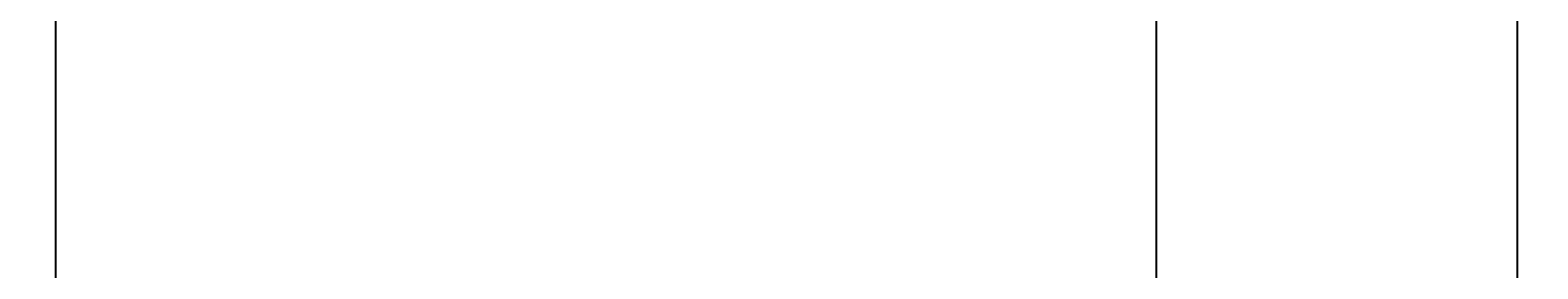
# Model space of a CAD drawing. Units: inches. Extents: x 35362 to 73946, y 43607 to 67532.
# Tile 77 of 134: x 50119 to 51337, y 46919 to 47112. Entities that reach past the tile are written whole.
import ezdxf

# ---------------------------------------------------------------- set-up
doc = ezdxf.new("R2010")
doc.units = ezdxf.units.IN
doc.header["$MEASUREMENT"] = 0
doc.layers.add('A-ANNO-DIMS', color=2, linetype='Continuous', lineweight=18)
doc.styles.get("Standard").update_dxf_attribs({"font": 'arial.ttf'})
doc.dimstyles.get("Standard").update_dxf_attribs({"dimtxt": 0.18, "dimasz": 0.18, "dimexe": 0.18, "dimexo": 0.0625, "dimgap": 0.09, "dimtad": 0, "dimtih": 1, "dimtoh": 1, "dimdec": 4, "dimzin": 0, "dimdsep": 46, "dimtxsty": 'Standard', "dimcen": 0.09, "dimadec": 0, "dimazin": 0, "dimtfac": 1, "dimtdec": 4, "dimtofl": 0, "dimtmove": 0, "dimatfit": 3, "dimfxl": 1, "dimtolj": 1, "dimtzin": 0, "dimarcsym": 0})

# ---------------------------------------------------------------- blocks, each defined once
blk = doc.blocks.new('*D11')
at = {"layer": 'A-ANNO-DIMS', "color": 0, "lineweight": -2, "transparency": 16777216}
for p, q in [((47978.7, 56028.8), (47978.7, 43606.7)), ((53109.8, 56028.8), (53109.8, 43606.7)), ((47978.8, 43606.9), (50543.9, 43606.9)), ((53109.6, 43606.9), (50544.6, 43606.9))]:
    blk.add_line(p, q, dxfattribs=at)
at = {"layer": 'A-ANNO-DIMS', "color": 0, "transparency": 16777216}
for points in [[(47978.8, 43606.9), (47978.8, 43606.8), (47978.7, 43606.9)], [(53109.6, 43606.9), (53109.6, 43606.8), (53109.8, 43606.9)]]:
    blk.add_solid(points, dxfattribs=at)
at = {"layer": 'Defpoints', "color": 0, "transparency": 16777216}
for p in [(47978.7, 56028.8), (53109.8, 56028.8), (53109.8, 43606.9)]:
    blk.add_point(p, dxfattribs=at)
at = {"layer": 'A-ANNO-DIMS', "color": 0, "transparency": 16777216, "insert": (50544.2, 43606.9), "char_height": 0.18, "attachment_point": 5}
blk.add_mtext('\\A1;5131', dxfattribs=at)
blk = doc.blocks.new('*D13')
at = {"layer": 'A-ANNO-DIMS', "color": 0, "lineweight": -2, "transparency": 16777216}
for p, q in [((48373.5, 51694), (48373.5, 43606.7)), ((51029, 51694), (51029, 43606.7)), ((48373.7, 43606.9), (49700.8, 43606.9)), ((51028.9, 43606.9), (49701.7, 43606.9))]:
    blk.add_line(p, q, dxfattribs=at)
at = {"layer": 'A-ANNO-DIMS', "color": 0, "transparency": 16777216}
for points in [[(48373.7, 43606.9), (48373.7, 43606.8), (48373.5, 43606.9)], [(51028.9, 43606.9), (51028.9, 43606.8), (51029, 43606.9)]]:
    blk.add_solid(points, dxfattribs=at)
at = {"layer": 'Defpoints', "color": 0, "transparency": 16777216}
for p in [(48373.5, 51694.1), (51029, 51694.1), (51029, 43606.9)]:
    blk.add_point(p, dxfattribs=at)
at = {"layer": 'A-ANNO-DIMS', "color": 0, "transparency": 16777216, "insert": (49701.3, 43606.9), "char_height": 0.18, "attachment_point": 5}
blk.add_mtext('\\A1;2655.6', dxfattribs=at)
blk = doc.blocks.new('*D17')
at = {"layer": 'A-ANNO-DIMS', "color": 0, "lineweight": -2, "transparency": 16777216}
for p, q in [((49923.3, 61293.2), (49923.3, 43606.7)), ((51913.9, 61293.2), (51913.9, 43606.7)), ((49923.5, 43606.9), (50918.2, 43606.9)), ((51913.8, 43606.9), (50919.1, 43606.9))]:
    blk.add_line(p, q, dxfattribs=at)
at = {"layer": 'A-ANNO-DIMS', "color": 0, "transparency": 16777216}
for points in [[(49923.5, 43606.9), (49923.5, 43606.8), (49923.3, 43606.9)], [(51913.8, 43606.9), (51913.8, 43606.8), (51913.9, 43606.9)]]:
    blk.add_solid(points, dxfattribs=at)
at = {"layer": 'Defpoints', "color": 0, "transparency": 16777216}
for p in [(49923.3, 61293.3), (51913.9, 61293.3), (51913.9, 43606.9)]:
    blk.add_point(p, dxfattribs=at)
at = {"layer": 'A-ANNO-DIMS', "color": 0, "transparency": 16777216, "insert": (50918.6, 43606.9), "char_height": 0.18, "attachment_point": 5}
blk.add_mtext('\\A1;1990.6', dxfattribs=at)
blk = doc.blocks.new('*D67')
at = {"layer": 'A-ANNO-DIMS', "color": 0, "lineweight": -2, "transparency": 16777216}
for p, q in [((56873.5, 53351.5), (35361.8, 53351.5)), ((35361.9, 53351.3), (35361.9, 49400.9)), ((35361.9, 45450.1), (35361.9, 49400.5)), ((53793.6, 45449.9), (35361.8, 45449.9))]:
    blk.add_line(p, q, dxfattribs=at)
at = {"layer": 'A-ANNO-DIMS', "color": 0, "transparency": 16777216}
for points in [[(35361.9, 53351.3), (35362, 53351.3), (35361.9, 53351.5)], [(35361.9, 45450.1), (35362, 45450.1), (35361.9, 45449.9)]]:
    blk.add_solid(points, dxfattribs=at)
at = {"layer": 'Defpoints', "color": 0, "transparency": 16777216}
for p in [(35361.9, 53351.5), (56873.6, 53351.5), (53793.6, 45449.9)]:
    blk.add_point(p, dxfattribs=at)
at = {"layer": 'A-ANNO-DIMS', "color": 0, "transparency": 16777216, "insert": (35361.9, 49400.7), "char_height": 0.18, "attachment_point": 5}
blk.add_mtext('\\A1;7901.6', dxfattribs=at)
blk = doc.blocks.new('*D90')
at = {"layer": 'A-ANNO-DIMS', "color": 0, "lineweight": -2, "transparency": 16777216}
for p, q in [((53707.7, 47291.3), (35361.8, 47291.3)), ((35361.9, 47291.1), (35361.9, 46710.3)), ((35361.9, 46129.1), (35361.9, 46709.9)), ((53793.6, 46128.9), (35361.8, 46128.9))]:
    blk.add_line(p, q, dxfattribs=at)
at = {"layer": 'A-ANNO-DIMS', "color": 0, "transparency": 16777216}
for points in [[(35361.9, 47291.1), (35362, 47291.1), (35361.9, 47291.3)], [(35361.9, 46129.1), (35362, 46129.1), (35361.9, 46128.9)]]:
    blk.add_solid(points, dxfattribs=at)
at = {"layer": 'Defpoints', "color": 0, "transparency": 16777216}
for p in [(53707.8, 47291.3), (35361.9, 46128.9), (53793.6, 46128.9)]:
    blk.add_point(p, dxfattribs=at)
at = {"layer": 'A-ANNO-DIMS', "color": 0, "transparency": 16777216, "insert": (35361.9, 46710.1), "char_height": 0.18, "attachment_point": 5}
blk.add_mtext('\\A1;1162.4', dxfattribs=at)
blk = doc.blocks.new('*D107')
at = {"layer": 'A-ANNO-DIMS', "color": 0, "lineweight": -2, "transparency": 16777216}
for p, q in [((50139.6, 59850), (50139.6, 43606.7)), ((51320.8, 59850), (51320.8, 43606.7)), ((50139.7, 43606.9), (50729.7, 43606.9)), ((51320.6, 43606.9), (50730.6, 43606.9))]:
    blk.add_line(p, q, dxfattribs=at)
at = {"layer": 'A-ANNO-DIMS', "color": 0, "transparency": 16777216}
for points in [[(50139.7, 43606.9), (50139.7, 43606.8), (50139.6, 43606.9)], [(51320.6, 43606.9), (51320.6, 43606.8), (51320.8, 43606.9)]]:
    blk.add_solid(points, dxfattribs=at)
at = {"layer": 'Defpoints', "color": 0, "transparency": 16777216}
for p in [(50139.6, 59850.1), (51320.8, 59850.1), (51320.8, 43606.9)]:
    blk.add_point(p, dxfattribs=at)
at = {"layer": 'A-ANNO-DIMS', "color": 0, "transparency": 16777216, "insert": (50730.2, 43606.9), "char_height": 0.18, "attachment_point": 5}
blk.add_mtext('\\A1;1181.3', dxfattribs=at)

msp = doc.modelspace()

# ---------------------------------------------------------------- dimensions: what is measured, and where the dimension line sits
at = {"layer": 'A-ANNO-DIMS'}
for base, p1, p2, override, picture, middle in [((51913.931, 43606.859), (49923.307, 61293.286), (51913.931, 61293.286), {"dimdec": 1, "dimlfac": 1, "dimrnd": 0, "dimzin": 0, "dimdsep": 46, "dimlunit": 2}, '*D17', (50918.619, 43606.859)), ((51320.8133, 43606.859), (50139.5627, 59850.0769), (51320.8133, 59850.0769), {"dimdec": 1, "dimlfac": 1, "dimrnd": 0, "dimzin": 0, "dimdsep": 46, "dimlunit": 2}, '*D107', (50730.188, 43606.859)), ((53109.76, 43606.859), (47978.665, 56028.836), (53109.76, 56028.836), {"dimdec": 0, "dimlfac": 1, "dimrnd": 0, "dimzin": 0, "dimdsep": 46, "dimlunit": 2}, '*D11', (50544.212, 43606.859)), ((51029.043, 43606.859), (48373.492, 51694.087), (51029.043, 51694.087), {"dimdec": 1, "dimlfac": 1, "dimrnd": 0, "dimzin": 0, "dimdsep": 46, "dimlunit": 2}, '*D13', (49701.267, 43606.859))]:
    dim = msp.add_linear_dim(base=base, p1=p1, p2=p2, dimstyle='Standard', override=override, dxfattribs=at)
    dim.commit()
    dim.dimension.update_dxf_attribs({"geometry": picture, "text_midpoint": middle})
for base, p1, p2, picture, middle in [((35361.949, 53351.529), (53793.638, 45449.894), (56873.602, 53351.529), '*D67', (35361.949, 49400.712)), ((35361.949, 46128.878), (53707.781, 47291.285), (53793.638, 46128.878), '*D90', (35361.949, 46710.081))]:
    dim = msp.add_linear_dim(base=base, p1=p1, p2=p2, angle=90, dimstyle='Standard', override={"dimdec": 1, "dimlfac": 1, "dimrnd": 0, "dimzin": 0, "dimdsep": 46, "dimlunit": 2}, dxfattribs=at)
    dim.commit()
    dim.dimension.update_dxf_attribs({"geometry": picture, "text_midpoint": middle})

doc.saveas('drawing.dxf')
